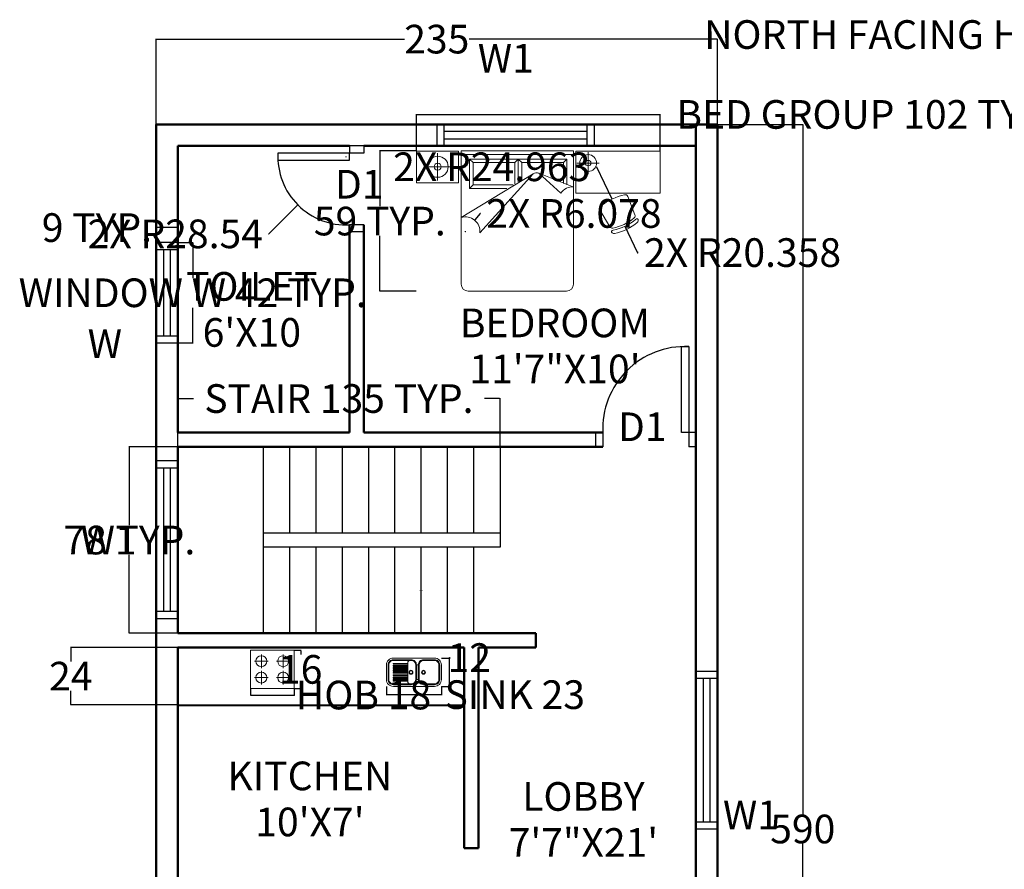
# Model space of a CAD drawing. Units: inches. Extents: x -15 to 810, y -55 to 662.
# Tile 2 of 3: x -15 to 397, y 302 to 658. Entities that reach past the tile are written whole.
import ezdxf
from ezdxf.enums import TextEntityAlignment as Align

# ---------------------------------------------------------------- set-up
doc = ezdxf.new("R2010")
doc.units = ezdxf.units.IN
doc.header["$MEASUREMENT"] = 0
for name, color, linetype, lineweight in [('A-ANNO-DIMS', 2, 'Continuous', 18), ('A-ANNO-TEXT', 1, 'Continuous', 25), ('A-AREA-IDEN', 1, 'Continuous', 25), ('A-DOOR', 2, 'Continuous', 25), ('A-EQPM', 8, 'Continuous', 18), ('A-FLOR-CASE', 8, 'Continuous', 25), ('A-FLOR-FIXT', 9, 'Continuous', 18), ('A-FLOR-STRS', 3, 'Continuous', 25), ('A-FURN', 8, 'Continuous', 18), ('A-GLAZ', 4, 'Continuous', 18), ('A-WALL', 6, 'Continuous', 50)]:
    doc.layers.add(name, color=color, linetype=linetype, lineweight=lineweight)
doc.layers.add('Layer3', color=4, linetype='Continuous')
doc.styles.get("Standard").update_dxf_attribs({"font": 'arial.ttf'})
doc.dimstyles.get("Standard").update_dxf_attribs({"dimtxt": 12, "dimasz": 0.18, "dimexe": 0.18, "dimexo": 0.0625, "dimgap": 0.09, "dimtad": 0, "dimtih": 1, "dimtoh": 1, "dimdec": 0, "dimzin": 0, "dimdsep": 46, "dimlunit": 4, "dimtxsty": 'Standard', "dimcen": 0.09, "dimadec": 0, "dimazin": 0, "dimtfac": 1, "dimtdec": 0, "dimtofl": 0, "dimtmove": 0, "dimatfit": 3, "dimfxl": 1, "dimtolj": 1, "dimtzin": 0, "dimarcsym": 0})

# ---------------------------------------------------------------- blocks, each defined once
blk = doc.blocks.new('A$C44EF7260')
for p, q in [((0, 1.998), (0.6, 1.998)), ((0, 1.548), (0, 1.998)), ((0.304, 1.579), (0.304, 1.971)), ((0.6, 1.998), (0.6, 1.548)), ((0.64, 2), (2.24, 2)), ((0.64, 0.1), (0.64, 2)), ((2.24, 2), (2.24, 0.1)), ((3.476, 1.998), (2.276, 1.998)), ((2.276, 1.998), (2.276, 1.398)), ((2.45, 1.671), (2.45, 1.985)), ((3.476, 1.398), (3.476, 1.998)), ((0.64, 1.95), (2.24, 1.95)), ((0.759, 1.884), (2.147, 1.884)), ((0.759, 1.884), (0.809, 1.834)), ((0.759, 1.467), (0.759, 1.884)), ((0.809, 1.834), (1.403, 1.834)), ((0.809, 1.517), (0.809, 1.834)), ((1.403, 1.834), (1.453, 1.884)), ((1.403, 1.834), (1.403, 1.53)), ((1.453, 1.884), (1.503, 1.834)), ((1.453, 1.884), (1.453, 1.558)), ((1.503, 1.834), (1.503, 1.586)), ((1.503, 1.834), (2.097, 1.834)), ((2.097, 1.834), (2.147, 1.884)), ((2.097, 1.834), (2.097, 1.535)), ((2.147, 1.884), (2.147, 1.519)), ((2.609, 1.828), (2.291, 1.828)), ((0.106, 1.775), (0.503, 1.775)), ((0.6, 1.548), (0, 1.548)), ((0.64, 1.05), (1.666, 1.676)), ((0.906, 0.833), (1.666, 1.676)), ((1.746, 1.684), (2.246, 1.486)), ((1.746, 1.684), (2.06, 1.397)), ((0.809, 1.517), (0.759, 1.467)), ((1.29, 1.467), (0.759, 1.467)), ((1.38, 1.517), (0.809, 1.517)), ((2.276, 1.398), (3.476, 1.398)), ((3.017, 1.352), (3.118, 1.091)), ((2.619, 1.162), (2.759, 0.919)), ((0.907, 0.845), (0.919, 0.845)), ((2.14, 0), (0.74, 0))]:
    blk.add_line(p, q)
for centre, radius in [((0.304, 1.775), 0.15), ((2.45, 1.828), 0.12), ((2.45, 1.828), 0.04), ((0.304, 1.775), 0.05)]:
    blk.add_circle(centre, radius)
for centre, radius, start, end in [((1.715, 1.589), 0.1, 71.7215, 119.0799), ((2.226, 1.289), 0.198, 84.1725, 146.9889), ((3.157, 0.547), 0.85, 102.6739, 128.3957), ((2.979, 1.337), 0.04, 21.3259, 102.6739), ((2.654, 1.182), 0.04, 128.3957, 209.9042), ((0.7, 0.852), 0.207, 354.6422, 106.9775), ((2.677, 1.551), 0.663, 280.7977, 310.4324), ((2.677, 1.551), 0.693, 280.6958, 310.5343), ((3.081, 1.077), 0.04, 310.4324, 21.3259), ((3.147, 1.002), 0.03, 70.2086, 130.5343), ((3.126, 1.01), 0.04, 309.6512, 20.6936), ((3.154, 1.02), 0.01, 20.6936, 70.2086), ((2.794, 0.939), 0.04, 209.9042, 280.7977), ((2.792, 0.847), 0.01, 161.0215, 210.5365), ((2.811, 0.841), 0.03, 100.6958, 161.0215), ((2.677, 1.551), 0.743, 281.5789, 309.6512), ((2.818, 0.862), 0.04, 210.5365, 281.5789), ((0.74, 0.1), 0.1, 180, 270), ((2.14, 0.1), 0.1, 270, 0)]:
    blk.add_arc(centre, radius, start, end)
blk = doc.blocks.new('A$C0A370B80')
for p, q in [((372, 413), (372, 83)), ((525, 375), (525, 121)), ((571, 375), (571, 121))]:
    blk.add_line(p, q)
for points in [[(962, 375), (962, 121, -0.414214), (841, 0), (121, 0, -0.414214), (0, 121), (0, 375, -0.414214), (121, 497), (841, 497, -0.414214)], [(434, 43), (412, 43), (313, 43), (121, 43, -0.414214), (43, 121), (43, 375, -0.414214), (121, 453), (313, 453), (412, 453), (434, 453, -0.414214), (512, 375), (512, 121, -0.414214)]]:
    blk.add_lwpolyline(points, format="xyb", close=True)
for points in [[(558, 121), (525, 121, -0.414214), (434, 30), (313, 30), (121, 30, -0.414214), (30, 121), (30, 375, -0.414214), (121, 467), (313, 467), (434, 467, -0.414214), (525, 375), (558, 375), (558, 121, 0.414214), (649, 30), (841, 30, 0.414214), (932, 121), (932, 375, 0.414214), (841, 467), (649, 467, 0.414214), (558, 375)], [(649, 453), (841, 453, -0.414214), (919, 375), (919, 121, -0.414214), (841, 43)]]:
    blk.add_lwpolyline(points, format="xyb")
for points in [[(366, 403), (366, 393), (120, 393), (120, 403)], [(366, 373), (366, 363), (120, 363), (120, 373)], [(366, 343), (366, 333), (120, 333), (120, 343)], [(366, 313), (366, 303), (120, 303), (120, 313)], [(366, 283), (366, 273), (120, 273), (120, 283)], [(366, 253), (366, 243), (120, 243), (120, 253)], [(366, 223), (366, 213), (120, 213), (120, 223)], [(366, 193), (366, 183), (120, 183), (120, 193)], [(366, 163), (366, 153), (120, 153), (120, 163)], [(366, 133), (366, 123), (120, 123), (120, 133)], [(366, 103), (366, 93), (120, 93), (120, 103)]]:
    blk.add_lwpolyline(points, close=True)
blk.add_lwpolyline([(649, 43), (841, 43)])
for centre, radius in [((430, 248), 34.6), ((430, 248), 25), ((649, 248), 34.6), ((649, 248), 25)]:
    blk.add_circle(centre, radius)
for centre, radius, start, end in [((412, 413), 40, 90, 180), ((649, 375), 78, 90, 180), ((412, 83), 40, 180, 270), ((649, 121), 78, 180, 270)]:
    blk.add_arc(centre, radius, start, end)
blk = doc.blocks.new('ESTUF-00')
for p, q in [((-0.375, 0.375), (-0.375, -0.325)), ((0.425, 0.375), (-0.375, 0.375)), ((0.425, -0.325), (0.425, 0.375)), ((-0.175, 0.05), (-0.175, 0.3)), ((0.225, 0.05), (0.225, 0.3)), ((-0.3, 0.175), (-0.05, 0.175)), ((-0.175, 0), (-0.175, -0.25)), ((0.1, 0.175), (0.35, 0.175)), ((0.225, 0), (0.225, -0.25)), ((-0.3, -0.125), (-0.05, -0.125)), ((0.1, -0.125), (0.35, -0.125)), ((-0.375, -0.325), (0.425, -0.325))]:
    blk.add_line(p, q)
for centre in [(-0.175, 0.175), (0.225, 0.175), (-0.175, -0.125), (0.225, -0.125)]:
    blk.add_circle(centre, 0.1)
blk = doc.blocks.new('v')
at = {"layer": 'Layer3'}
for p, q in [((0, 0), (0, -9)), ((39, 0), (3, 0)), ((3, 0), (3, -9)), ((39, -9), (39, 0)), ((42, -9), (42, 0)), ((39, -3), (3, -3)), ((3, -6), (39, -6)), ((3, -9), (39, -9))]:
    blk.add_line(p, q, dxfattribs=at)
blk = doc.blocks.new('gh')
at = {"layer": 'Layer3'}
for p, q in [((0, 0), (0, -9)), ((63, 0), (3, 0)), ((3, 0), (3, -9)), ((63, -9), (63, 0)), ((66, -9), (66, 0)), ((63, -3), (3, -3)), ((3, -6), (63, -6)), ((3, -9), (63, -9))]:
    blk.add_line(p, q, dxfattribs=at)
blk = doc.blocks.new('DOOR-SWING-30IN')
for p, q in [((36.04, 36), (30.04, 36)), ((30.04, 36), (30.04, 33)), ((36.04, 33), (30.04, 33)), ((36.04, 36), (36.04, 33)), ((36.04, 3), (30.04, 3)), ((36.04, 0), (30.04, 0))]:
    blk.add_line(p, q)
blk.add_lwpolyline([(30.04, 33), (0.04, 33), (0.04, 30), (30.04, 30)], close=True)
blk.add_arc((28.54, 31.5), 28.54, 176.9872, 273.0128)
blk = doc.blocks.new('DOOR-SWING-36IN')
for p, q in [((0, 6), (0, 0)), ((3, 6), (3, 0)), ((39, 6), (39, 0)), ((42, 6), (39, 6)), ((42, 6), (42, 0)), ((42, 0), (39, 0))]:
    blk.add_line(p, q)
blk.add_lwpolyline([(39, 6), (36, 6), (36, 42), (39, 42)], close=True)
blk.add_arc((37.5, 7.5), 34.53, 87.5104, 182.4896)
blk = doc.blocks.new('STAIR-HALF-TURN')
for p, q in [((0, 78), (135, 78)), ((0, 0), (0, 78)), ((36, 0), (36, 78)), ((47, 42), (47, 78)), ((58, 42), (58, 78)), ((69, 42), (69, 78)), ((80, 42), (80, 78)), ((91, 42), (91, 78)), ((102, 42), (102, 78)), ((113, 42), (113, 78)), ((124, 42), (124, 78)), ((135, 78), (135, 36)), ((36, 42), (135, 42)), ((135, 36), (36, 36)), ((47, 0), (47, 36)), ((58, 0), (58, 36)), ((69, 0), (69, 36)), ((80, 0), (80, 36)), ((91, 0), (91, 36)), ((102, 0), (102, 36)), ((113, 0), (113, 36)), ((124, 0), (124, 36)), ((124, 0), (0, 0))]:
    blk.add_line(p, q)
blk.add_lwpolyline([(124, 60, 0, 0, 0), (11.12, 60, 0, 0, 0), (11.12, 18.31, 0, 0, 0), (69, 18, 12, 0, 0), (102, 18, 0, 0, 0)], format="xyseb")
blk = doc.blocks.new('*D14')
at = {"layer": 'A-ANNO-DIMS', "color": 0, "lineweight": -2, "transparency": 16777216}
for p, q in [((51.25, 564.24), (57.67, 564.24)), ((57.49, 564.06), (57.49, 549.54)), ((57.49, 522.42), (57.49, 536.95)), ((51.25, 522.24), (57.67, 522.24))]:
    blk.add_line(p, q, dxfattribs=at)
at = {"layer": 'A-ANNO-DIMS', "color": 0, "transparency": 16777216}
for points in [[(57.46, 564.06), (57.52, 564.06), (57.49, 564.24)], [(57.46, 522.42), (57.52, 522.42), (57.49, 522.24)]]:
    blk.add_solid(points, dxfattribs=at)
at = {"layer": 'Defpoints', "color": 0, "transparency": 16777216}
for p in [(51.19, 564.24), (57.49, 564.24), (51.19, 522.24)]:
    blk.add_point(p, dxfattribs=at)
at = {"layer": 'A-ANNO-DIMS', "color": 0, "transparency": 16777216, "insert": (57.49, 543.24), "char_height": 12, "attachment_point": 5}
blk.add_mtext('\\A1;WINDOW W 42 TYP.', dxfattribs=at)
blk = doc.blocks.new('*D15')
at = {"layer": 'A-ANNO-DIMS', "color": 0, "lineweight": -2, "transparency": 16777216}
for p, q in [((42.19, 570.54), (42.01, 570.54)), ((42.19, 564.31), (42.19, 570.72)), ((51.01, 570.54), (42.37, 570.54)), ((51.19, 564.31), (51.19, 570.72))]:
    blk.add_line(p, q, dxfattribs=at)
at = {"layer": 'A-ANNO-DIMS', "color": 0, "transparency": 16777216}
for points in [[(42.37, 570.57), (42.37, 570.51), (42.19, 570.54)], [(51.01, 570.57), (51.01, 570.51), (51.19, 570.54)]]:
    blk.add_solid(points, dxfattribs=at)
at = {"layer": 'Defpoints', "color": 0, "transparency": 16777216}
for p in [(42.19, 570.54), (42.19, 564.24), (51.19, 564.24)]:
    blk.add_point(p, dxfattribs=at)
at = {"layer": 'A-ANNO-DIMS', "color": 0, "transparency": 16777216, "insert": (17.37, 570.54), "char_height": 12, "attachment_point": 5}
blk.add_mtext('\\A1;9 TYP.', dxfattribs=at)
blk = doc.blocks.new('*D16')
at = {"layer": 'A-ANNO-DIMS', "color": 0, "lineweight": -2, "transparency": 16777216}
for p, q in [((51.19, 478.77), (51.19, 499.13)), ((51.37, 498.95), (57.75, 498.95)), ((186.01, 498.95), (179.63, 498.95)), ((186.19, 478.77), (186.19, 499.13))]:
    blk.add_line(p, q, dxfattribs=at)
at = {"layer": 'A-ANNO-DIMS', "color": 0, "transparency": 16777216}
for points in [[(51.37, 498.98), (51.37, 498.92), (51.19, 498.95)], [(186.01, 498.98), (186.01, 498.92), (186.19, 498.95)]]:
    blk.add_solid(points, dxfattribs=at)
at = {"layer": 'Defpoints', "color": 0, "transparency": 16777216}
for p in [(186.19, 498.95), (51.19, 478.7), (186.19, 478.7)]:
    blk.add_point(p, dxfattribs=at)
at = {"layer": 'A-ANNO-DIMS', "color": 0, "transparency": 16777216, "insert": (118.69, 498.95), "char_height": 12, "attachment_point": 5}
blk.add_mtext('\\A1;STAIR 135 TYP.', dxfattribs=at)
blk = doc.blocks.new('*D17')
at = {"layer": 'A-ANNO-DIMS', "color": 0, "lineweight": -2, "transparency": 16777216}
for p, q in [((51.12, 478.7), (30.76, 478.7)), ((30.94, 478.52), (30.94, 445.92)), ((30.94, 400.88), (30.94, 433.49)), ((51.12, 400.7), (30.76, 400.7))]:
    blk.add_line(p, q, dxfattribs=at)
at = {"layer": 'A-ANNO-DIMS', "color": 0, "transparency": 16777216}
for points in [[(30.91, 478.52), (30.97, 478.52), (30.94, 478.7)], [(30.91, 400.88), (30.97, 400.88), (30.94, 400.7)]]:
    blk.add_solid(points, dxfattribs=at)
at = {"layer": 'Defpoints', "color": 0, "transparency": 16777216}
for p in [(30.94, 478.7), (51.19, 478.7), (51.19, 400.7)]:
    blk.add_point(p, dxfattribs=at)
at = {"layer": 'A-ANNO-DIMS', "color": 0, "transparency": 16777216, "insert": (30.94, 439.7), "char_height": 12, "attachment_point": 5}
blk.add_mtext('\\A1;78 TYP.', dxfattribs=at)
blk = doc.blocks.new('*D18')
at = {"layer": 'A-ANNO-DIMS', "color": 0, "lineweight": -2, "transparency": 16777216}
for p, q in [((151.13, 602.68), (151.13, 618.1)), ((151.31, 617.92), (252.98, 617.92)), ((253.16, 602.68), (253.16, 618.1)), ((253.16, 617.92), (253.34, 617.92))]:
    blk.add_line(p, q, dxfattribs=at)
at = {"layer": 'A-ANNO-DIMS', "color": 0, "transparency": 16777216}
for points in [[(151.31, 617.95), (151.31, 617.89), (151.13, 617.92)], [(252.98, 617.95), (252.98, 617.89), (253.16, 617.92)]]:
    blk.add_solid(points, dxfattribs=at)
at = {"layer": 'Defpoints', "color": 0, "transparency": 16777216}
for p in [(253.16, 617.92), (151.13, 602.62), (253.16, 602.62)]:
    blk.add_point(p, dxfattribs=at)
at = {"layer": 'A-ANNO-DIMS', "color": 0, "transparency": 16777216, "insert": (339.66, 617.92), "char_height": 12, "attachment_point": 5}
blk.add_mtext('\\A1;BED GROUP 102 TYP.', dxfattribs=at)
blk = doc.blocks.new('*D19')
at = {"layer": 'A-ANNO-DIMS', "color": 0, "lineweight": -2, "transparency": 16777216}
for p, q in [((151.06, 602.62), (135.64, 602.62)), ((135.82, 602.44), (135.82, 579.48)), ((135.82, 544.08), (135.82, 567.04)), ((151.06, 543.9), (135.64, 543.9))]:
    blk.add_line(p, q, dxfattribs=at)
at = {"layer": 'A-ANNO-DIMS', "color": 0, "transparency": 16777216}
for points in [[(135.79, 602.44), (135.85, 602.44), (135.82, 602.62)], [(135.79, 544.08), (135.85, 544.08), (135.82, 543.9)]]:
    blk.add_solid(points, dxfattribs=at)
at = {"layer": 'Defpoints', "color": 0, "transparency": 16777216}
for p in [(135.82, 602.62), (151.13, 602.62), (151.13, 543.9)]:
    blk.add_point(p, dxfattribs=at)
at = {"layer": 'A-ANNO-DIMS', "color": 0, "transparency": 16777216, "insert": (135.82, 573.26), "char_height": 12, "attachment_point": 5}
blk.add_mtext('\\A1;59 TYP.', dxfattribs=at)
blk = doc.blocks.new('*D30')
at = {"layer": 'A-ANNO-DIMS', "color": 0, "lineweight": -2, "transparency": 16777216}
for p, q in [((138.6, 378.34), (138.6, 374.77)), ((161.62, 378.34), (161.62, 374.77)), ((138.78, 374.95), (161.44, 374.95)), ((161.62, 374.95), (161.8, 374.95))]:
    blk.add_line(p, q, dxfattribs=at)
at = {"layer": 'A-ANNO-DIMS', "color": 0, "transparency": 16777216}
for points in [[(138.78, 374.98), (138.78, 374.92), (138.6, 374.95)], [(161.44, 374.98), (161.44, 374.92), (161.62, 374.95)]]:
    blk.add_solid(points, dxfattribs=at)
at = {"layer": 'Defpoints', "color": 0, "transparency": 16777216}
for p in [(138.6, 378.4), (161.62, 378.4), (161.62, 374.95)]:
    blk.add_point(p, dxfattribs=at)
at = {"layer": 'A-ANNO-DIMS', "color": 0, "transparency": 16777216, "insert": (192.35, 374.95), "char_height": 12, "attachment_point": 5}
blk.add_mtext('\\A1;SINK 23', dxfattribs=at)
blk = doc.blocks.new('*D31')
at = {"layer": 'A-ANNO-DIMS', "color": 0, "lineweight": -2, "transparency": 16777216}
for p, q in [((161.68, 390.29), (165.25, 390.29)), ((165.07, 390.29), (165.07, 390.47)), ((165.07, 390.47), (165.25, 390.47)), ((165.07, 378.58), (165.07, 390.11)), ((161.68, 378.4), (165.25, 378.4))]:
    blk.add_line(p, q, dxfattribs=at)
at = {"layer": 'A-ANNO-DIMS', "color": 0, "transparency": 16777216}
for points in [[(165.04, 390.11), (165.1, 390.11), (165.07, 390.29)], [(165.04, 378.58), (165.1, 378.58), (165.07, 378.4)]]:
    blk.add_solid(points, dxfattribs=at)
at = {"layer": 'Defpoints', "color": 0, "transparency": 16777216}
for p in [(161.62, 390.29), (165.07, 390.29), (161.62, 378.4)]:
    blk.add_point(p, dxfattribs=at)
at = {"layer": 'A-ANNO-DIMS', "color": 0, "transparency": 16777216, "insert": (173.31, 390.47), "char_height": 12, "attachment_point": 5}
blk.add_mtext('\\A1;12', dxfattribs=at)
blk = doc.blocks.new('*D32')
at = {"layer": 'A-ANNO-DIMS', "color": 0, "lineweight": -2, "transparency": 16777216}
for p, q in [((81.65, 377.48), (81.65, 374.61)), ((99.94, 377.48), (99.94, 374.61)), ((81.83, 374.79), (99.76, 374.79)), ((99.94, 374.79), (100.12, 374.79))]:
    blk.add_line(p, q, dxfattribs=at)
at = {"layer": 'A-ANNO-DIMS', "color": 0, "transparency": 16777216}
for points in [[(81.83, 374.82), (81.83, 374.76), (81.65, 374.79)], [(99.76, 374.82), (99.76, 374.76), (99.94, 374.79)]]:
    blk.add_solid(points, dxfattribs=at)
at = {"layer": 'Defpoints', "color": 0, "transparency": 16777216}
for p in [(81.65, 377.54), (99.94, 377.54), (99.94, 374.79)]:
    blk.add_point(p, dxfattribs=at)
at = {"layer": 'A-ANNO-DIMS', "color": 0, "transparency": 16777216, "insert": (128.99, 374.79), "char_height": 12, "attachment_point": 5}
blk.add_mtext('\\A1;HOB 18', dxfattribs=at)
blk = doc.blocks.new('*D33')
at = {"layer": 'A-ANNO-DIMS', "color": 0, "lineweight": -2, "transparency": 16777216}
for p, q in [((100, 393.55), (102.87, 393.55)), ((102.69, 393.37), (102.69, 391.76)), ((102.69, 377.72), (102.69, 379.33)), ((100, 377.54), (102.87, 377.54))]:
    blk.add_line(p, q, dxfattribs=at)
at = {"layer": 'A-ANNO-DIMS', "color": 0, "transparency": 16777216}
for points in [[(102.66, 393.37), (102.72, 393.37), (102.69, 393.55)], [(102.66, 377.72), (102.72, 377.72), (102.69, 377.54)]]:
    blk.add_solid(points, dxfattribs=at)
at = {"layer": 'Defpoints', "color": 0, "transparency": 16777216}
for p in [(99.94, 393.55), (102.69, 393.55), (99.94, 377.54)]:
    blk.add_point(p, dxfattribs=at)
at = {"layer": 'A-ANNO-DIMS', "color": 0, "transparency": 16777216, "insert": (102.69, 385.54), "char_height": 12, "attachment_point": 5}
blk.add_mtext('\\A1;16', dxfattribs=at)
blk = doc.blocks.new('*D34')
at = {"layer": 'A-ANNO-DIMS', "color": 0, "lineweight": -2, "transparency": 16777216}
for p, q in [((42.19, 613.77), (42.19, 649.63)), ((42.37, 649.45), (146.19, 649.45)), ((277.01, 649.45), (173.18, 649.45)), ((277.19, 613.77), (277.19, 649.63))]:
    blk.add_line(p, q, dxfattribs=at)
at = {"layer": 'A-ANNO-DIMS', "color": 0, "transparency": 16777216}
for points in [[(42.37, 649.48), (42.37, 649.42), (42.19, 649.45)], [(277.01, 649.48), (277.01, 649.42), (277.19, 649.45)]]:
    blk.add_solid(points, dxfattribs=at)
at = {"layer": 'Defpoints', "color": 0, "transparency": 16777216}
for p in [(277.19, 649.45), (42.19, 613.7), (277.19, 613.7)]:
    blk.add_point(p, dxfattribs=at)
at = {"layer": 'A-ANNO-DIMS', "color": 0, "transparency": 16777216, "insert": (159.69, 649.45), "char_height": 12, "attachment_point": 5}
blk.add_mtext('\\A1;235', dxfattribs=at)
blk = doc.blocks.new('*D35')
at = {"layer": 'A-ANNO-DIMS', "color": 0, "lineweight": -2, "transparency": 16777216}
for p, q in [((277.25, 613.7), (313.12, 613.7)), ((312.94, 613.52), (312.94, 324.92)), ((312.94, 23.88), (312.94, 312.49)), ((277.25, 23.7), (313.12, 23.7))]:
    blk.add_line(p, q, dxfattribs=at)
at = {"layer": 'A-ANNO-DIMS', "color": 0, "transparency": 16777216}
for points in [[(312.91, 613.52), (312.97, 613.52), (312.94, 613.7)], [(312.91, 23.88), (312.97, 23.88), (312.94, 23.7)]]:
    blk.add_solid(points, dxfattribs=at)
at = {"layer": 'Defpoints', "color": 0, "transparency": 16777216}
for p in [(277.19, 613.7), (312.94, 613.7), (277.19, 23.7)]:
    blk.add_point(p, dxfattribs=at)
at = {"layer": 'A-ANNO-DIMS', "color": 0, "transparency": 16777216, "insert": (312.94, 318.7), "char_height": 12, "attachment_point": 5}
blk.add_mtext('\\A1;590', dxfattribs=at)
blk = doc.blocks.new('*D50')
at = {"layer": 'A-ANNO-DIMS', "color": 0, "lineweight": -2, "transparency": 16777216}
for p, q in [((51.12, 394.7), (6.26, 394.7)), ((6.44, 394.52), (6.44, 388.82)), ((6.44, 370.88), (6.44, 376.59)), ((51.12, 370.7), (6.26, 370.7))]:
    blk.add_line(p, q, dxfattribs=at)
at = {"layer": 'A-ANNO-DIMS', "color": 0, "transparency": 16777216}
for points in [[(6.41, 394.52), (6.47, 394.52), (6.44, 394.7)], [(6.41, 370.88), (6.47, 370.88), (6.44, 370.7)]]:
    blk.add_solid(points, dxfattribs=at)
at = {"layer": 'Defpoints', "color": 0, "transparency": 16777216}
for p in [(6.44, 394.7), (51.19, 394.7), (51.19, 370.7)]:
    blk.add_point(p, dxfattribs=at)
at = {"layer": 'A-ANNO-DIMS', "color": 0, "transparency": 16777216, "insert": (6.44, 382.7), "char_height": 12, "attachment_point": 5}
blk.add_mtext('\\A1;24', dxfattribs=at)
blk = doc.blocks.new('*D57')
at = {"layer": 'A-ANNO-DIMS', "color": 0, "lineweight": -2, "transparency": 16777216}
for p, q in [((121.6, 600.2), (121.78, 600.2)), ((121.69, 600.11), (121.69, 600.29)), ((89.4, 567.91), (101.38, 579.9)), ((89.22, 567.91), (89.4, 567.91))]:
    blk.add_line(p, q, dxfattribs=at)
at = {"layer": 'A-ANNO-DIMS', "color": 0, "transparency": 16777216}
blk.add_solid([(101.36, 579.92), (101.4, 579.87), (101.51, 580.02)], dxfattribs=at)
at = {"layer": 'Defpoints', "color": 0, "transparency": 16777216}
for p in [(121.69, 600.2), (101.51, 580.02)]:
    blk.add_point(p, dxfattribs=at)
at = {"layer": 'A-ANNO-DIMS', "color": 0, "transparency": 16777216, "insert": (50.17, 567.91), "char_height": 12, "attachment_point": 5}
blk.add_mtext('\\A1;2X R28.54', dxfattribs=at)
blk = doc.blocks.new('*D59')
at = {"layer": 'A-ANNO-DIMS', "color": 0, "lineweight": -2, "transparency": 16777216}
for p, q in [((226.42, 595.99), (226.6, 595.99)), ((226.6, 595.99), (232.98, 582.64)), ((243.72, 559.95), (243.9, 559.95)), ((243.81, 559.86), (243.81, 560.04))]:
    blk.add_line(p, q, dxfattribs=at)
at = {"layer": 'A-ANNO-DIMS', "color": 0, "transparency": 16777216}
blk.add_solid([(233, 582.65), (232.95, 582.62), (233.05, 582.47)], dxfattribs=at)
at = {"layer": 'Defpoints', "color": 0, "transparency": 16777216}
for p in [(233.05, 582.47), (243.81, 559.95)]:
    blk.add_point(p, dxfattribs=at)
at = {"layer": 'A-ANNO-DIMS', "color": 0, "transparency": 16777216, "insert": (182.68, 595.99), "char_height": 12, "attachment_point": 5}
blk.add_mtext('\\A1;2X R24.963', dxfattribs=at)
blk = doc.blocks.new('*D61')
at = {"layer": 'A-ANNO-DIMS', "color": 0, "lineweight": -2, "transparency": 16777216}
for p, q in [((229.62, 589.45), (229.8, 589.45)), ((229.71, 589.36), (229.71, 589.54)), ((243.79, 560.07), (238.59, 570.93)), ((243.97, 560.07), (243.79, 560.07))]:
    blk.add_line(p, q, dxfattribs=at)
at = {"layer": 'A-ANNO-DIMS', "color": 0, "transparency": 16777216}
blk.add_solid([(238.61, 570.94), (238.56, 570.91), (238.51, 571.09)], dxfattribs=at)
at = {"layer": 'Defpoints', "color": 0, "transparency": 16777216}
for p in [(229.71, 589.45), (238.51, 571.09)]:
    blk.add_point(p, dxfattribs=at)
at = {"layer": 'A-ANNO-DIMS', "color": 0, "transparency": 16777216, "insert": (287.72, 560.07), "char_height": 12, "attachment_point": 5}
blk.add_mtext('\\A1;2X R20.358', dxfattribs=at)
blk = doc.blocks.new('*D63')
at = {"layer": 'A-ANNO-DIMS', "color": 0, "lineweight": -2, "transparency": 16777216}
for p, q in [((177.83, 576.45), (175.64, 573.77)), ((178.01, 576.45), (177.83, 576.45)), ((171.68, 568.82), (171.68, 569)), ((171.59, 568.91), (171.77, 568.91))]:
    blk.add_line(p, q, dxfattribs=at)
at = {"layer": 'A-ANNO-DIMS', "color": 0, "transparency": 16777216}
blk.add_solid([(175.61, 573.78), (175.66, 573.75), (175.52, 573.63)], dxfattribs=at)
at = {"layer": 'Defpoints', "color": 0, "transparency": 16777216}
for p in [(175.52, 573.63), (171.68, 568.91)]:
    blk.add_point(p, dxfattribs=at)
at = {"layer": 'A-ANNO-DIMS', "color": 0, "transparency": 16777216, "insert": (217.09, 576.45), "char_height": 12, "attachment_point": 5}
blk.add_mtext('\\A1;2X R6.078', dxfattribs=at)

msp = doc.modelspace()

# ---------------------------------------------------------------- linework, layer by layer
at = {"layer": 'A-FLOR-CASE'}
for p, q in [((51.1872, 370.7034), (171.1872, 370.7034)), ((51.1872, 370.4034), (171.1872, 370.4034))]:
    msp.add_line(p, q, dxfattribs=at)
at = {"layer": 'A-WALL'}
for p, q in [((268.1872, 32.7034), (268.1872, 613.7034)), ((51.1872, 604.7034), (51.1872, 484.7034)), ((123.1872, 604.7034), (51.1872, 604.7034)), ((268.1872, 604.7034), (129.1872, 604.7034)), ((268.1872, 484.7034), (268.1872, 604.7034)), ((123.1872, 571.7034), (123.1872, 484.7034)), ((129.1872, 571.7034), (129.1872, 484.7034)), ((123.1872, 484.7034), (51.1872, 484.7034)), ((229.1872, 484.7034), (129.1872, 484.7034)), ((51.1872, 478.7034), (51.1872, 400.7034)), ((229.1872, 478.7034), (51.1872, 478.7034)), ((268.1872, 214.7034), (268.1872, 478.7034)), ((51.1872, 400.7034), (201.1872, 400.7034)), ((201.1872, 394.7034), (201.1872, 400.7034)), ((51.1872, 394.7034), (171.1872, 394.7034)), ((51.1872, 394.7034), (51.1872, 214.7034)), ((171.1872, 394.7034), (171.1872, 310.7034)), ((177.1872, 394.7034), (177.1872, 310.7034)), ((177.1872, 394.7034), (201.1872, 394.7034)), ((171.1872, 310.7034), (177.1872, 310.7034))]:
    msp.add_line(p, q, dxfattribs=at)
msp.add_lwpolyline([(265.1872, 23.7034), (277.1872, 23.7034), (277.1872, 613.7034), (42.1872, 613.7034), (42.1872, 23.7034), (229.1872, 23.7034)], dxfattribs=at)

# ---------------------------------------------------------------- block references
at = {"layer": 'A-DOOR'}
for name, p in [('DOOR-SWING-30IN', (93.148, 568.703)), ('DOOR-SWING-36IN', (226.187, 478.703))]:
    msp.add_blockref(name, p, dxfattribs=at)
at = {"layer": 'A-EQPM', "xscale": 22.86913632663783, "yscale": 22.86913632663783, "zscale": 22.86913632663783}
msp.add_blockref('ESTUF-00', (90.2226, 384.9705), dxfattribs=at)
at = {"layer": 'A-FLOR-FIXT', "xscale": 0.023919604723985, "yscale": 0.023919604723985, "zscale": 0.023919604723985}
msp.add_blockref('A$C0A370B80', (138.6017, 378.4048), dxfattribs=at)
at = {"layer": 'A-FLOR-STRS'}
msp.add_blockref('STAIR-HALF-TURN', (51.187, 400.703), dxfattribs=at)
at = {"layer": 'A-FURN', "xscale": 29.35705846695051, "yscale": 29.35705846695051, "zscale": 29.35705846695051}
msp.add_blockref('A$C44EF7260', (151.1269, 543.9012), dxfattribs=at)
at = {"layer": 'A-GLAZ'}
msp.add_blockref('gh', (159.6872, 613.7034), dxfattribs=at)
at = {"layer": 'A-GLAZ', "rotation": 90}
for name, p in [('v', (42.1872, 522.244)), ('gh', (42.1872, 406.8559)), ('gh', (268.1872, 318.7034))]:
    msp.add_blockref(name, p, dxfattribs=at)

# ---------------------------------------------------------------- texts
at = {"layer": 'A-ANNO-TEXT'}
for s, p in [('NORTH FACING HOUSE', (359.6923, 645.3791)), ('W1', (188.5775, 635.4492)), ('D1', (127.2215, 582.6817)), ('W', (20.6949, 515.8777)), ('D1', (245.7297, 481.1314)), ('W1', (22.288, 433.6508)), ('W1', (291.2444, 318.6196))]:
    msp.add_text(s, height=12, dxfattribs=at).set_placement(p, align=Align.CENTER)
at = {"layer": 'A-AREA-IDEN'}
for s, p in [('TOILET', (82.2398, 539.9157)), ('BEDROOM', (209.1682, 524.6153)), ("6'X10", (82.2398, 520.6388)), ('11\'7"X10\'', (209.1682, 505.3384)), ('KITCHEN', (106.5633, 334.9327)), ('LOBBY', (221.0815, 326.325)), ("10'X7'", (106.5633, 315.6558)), ('7\'7"X21\'', (221.0815, 307.0481))]:
    msp.add_text(s, height=12, dxfattribs=at).set_placement(p, align=Align.CENTER)

# ---------------------------------------------------------------- dimensions: what is measured, and where the dimension line sits
at = {"layer": 'A-ANNO-DIMS'}
dim = msp.add_linear_dim(base=(277.1872, 649.4534), p1=(42.1872, 613.7034), p2=(277.1872, 613.7034), dimstyle='Standard', override={"dimdec": 0, "dimlfac": 1, "dimrnd": 0, "dimzin": 0, "dimdsep": 46, "dimlunit": 2}, dxfattribs=at)
dim.commit()
dim.dimension.update_dxf_attribs({"geometry": '*D34', "text_midpoint": (159.6872, 649.4534)})
for base, p1, p2, text, picture, middle in [((253.1593, 617.9222), (151.1262, 602.6172), (253.1593, 602.6172), 'BED GROUP <> TYP.', '*D18', (339.6599, 617.9222)), ((186.1872, 498.9534), (51.1872, 478.7034), (186.1872, 478.7034), 'STAIR <> TYP.', '*D16', (118.6872, 498.9534)), ((99.942, 374.7937), (81.6467, 377.538), (99.942, 377.538), 'HOB <>', '*D32', (128.9883, 374.7937)), ((161.6219, 374.9518), (138.6017, 378.4048), (161.6219, 378.4048), 'SINK <>', '*D30', (192.3503, 374.9518))]:
    dim = msp.add_linear_dim(base=base, p1=p1, p2=p2, text=text, dimstyle='Standard', override={"dimdec": 0, "dimlfac": 1, "dimrnd": 0, "dimzin": 0, "dimdsep": 46, "dimlunit": 2}, dxfattribs=at)
    dim.commit()
    dim.dimension.update_dxf_attribs({"geometry": picture, "text_midpoint": middle})
for center, mpoint, override, picture, middle in [((243.8144, 559.9483), (233.0541, 582.4727), {"dimdec": 3, "dimlfac": 1, "dimrnd": 0, "dimzin": 0, "dimdsep": 46, "dimlunit": 2}, '*D59', (182.6826, 595.9874)), ((121.6872, 600.2034), (101.5069, 580.0229), {"dimdec": 2, "dimlfac": 1, "dimrnd": 0, "dimzin": 0, "dimdsep": 46, "dimlunit": 2}, '*D57', (50.1696, 567.9145)), ((171.681, 568.9149), (175.5217, 573.6256), {"dimdec": 3, "dimlfac": 1, "dimrnd": 0, "dimzin": 0, "dimdsep": 46, "dimlunit": 2}, '*D63', (217.092, 576.452)), ((229.7085, 589.4461), (238.51, 571.0891), {"dimdec": 3, "dimlfac": 1, "dimrnd": 0, "dimzin": 0, "dimdsep": 46, "dimlunit": 2}, '*D61', (287.7184, 560.0749))]:
    dim = msp.add_radius_dim(center=center, mpoint=mpoint, text='2X <>', dimstyle='Standard', override=override, dxfattribs=at)
    dim.commit()
    dim.dimension.update_dxf_attribs({"geometry": picture, "text_midpoint": middle, "dimtype": 164})
for base, p1, p2, picture, middle in [((312.9372, 613.7034), (277.1872, 23.7034), (277.1872, 613.7034), '*D35', (312.9372, 318.7034)), ((165.075, 390.2928), (161.6219, 378.4048), (161.6219, 390.2928), '*D31', (173.3136, 390.4728)), ((6.4372, 394.7034), (51.1872, 370.7034), (51.1872, 394.7034), '*D50', (6.4372, 382.7034)), ((102.6863, 393.5464), (99.942, 377.538), (99.942, 393.5464), '*D33', (102.6863, 385.5422))]:
    dim = msp.add_linear_dim(base=base, p1=p1, p2=p2, angle=90, dimstyle='Standard', override={"dimdec": 0, "dimlfac": 1, "dimrnd": 0, "dimzin": 0, "dimdsep": 46, "dimlunit": 2}, dxfattribs=at)
    dim.commit()
    dim.dimension.update_dxf_attribs({"geometry": picture, "text_midpoint": middle})
for base, p1, p2, angle, text, picture, middle in [((135.8212, 602.6172), (151.1262, 543.9031), (151.1262, 602.6172), 90, '<> TYP.', '*D19', (135.8212, 573.2601)), ((42.1872, 570.544), (51.1872, 564.244), (42.1872, 564.244), 180, '<> TYP.', '*D15', (17.3729, 570.544)), ((57.4872, 564.244), (51.1872, 522.244), (51.1872, 564.244), 90, 'WINDOW W <> TYP.', '*D14', (57.4872, 543.244)), ((30.9372, 478.7034), (51.1872, 400.7034), (51.1872, 478.7034), 90, '<> TYP.', '*D17', (30.9372, 439.7034))]:
    dim = msp.add_linear_dim(base=base, p1=p1, p2=p2, angle=angle, text=text, dimstyle='Standard', override={"dimdec": 0, "dimlfac": 1, "dimrnd": 0, "dimzin": 0, "dimdsep": 46, "dimlunit": 2}, dxfattribs=at)
    dim.commit()
    dim.dimension.update_dxf_attribs({"geometry": picture, "text_midpoint": middle})

doc.saveas('drawing.dxf')
